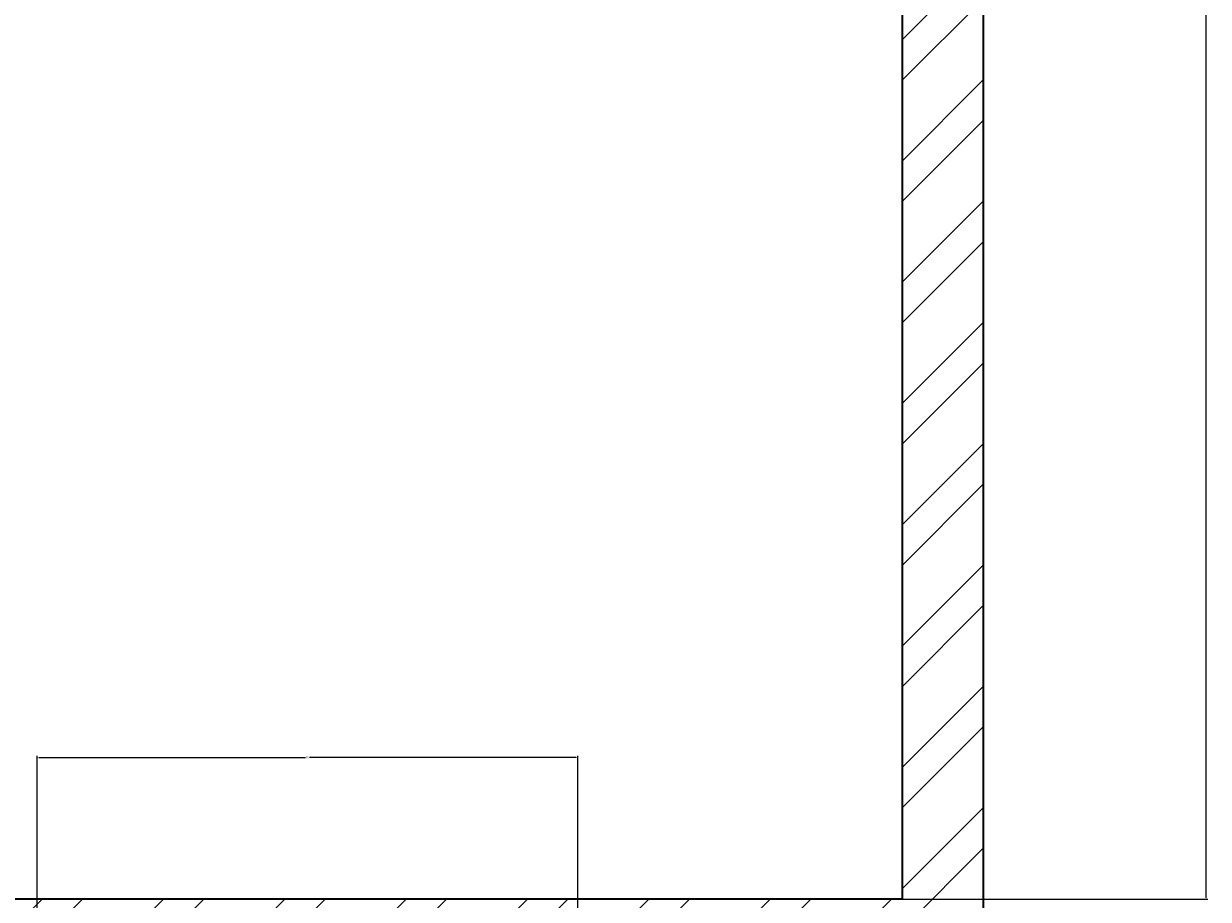
# Model space of a CAD drawing. Units: inches. Extents: x 2166 to 3588, y 1959 to 2628.
# Tile 12 of 13: x 3457 to 3588, y 2112 to 2209. Entities that reach past the tile are written whole.
import ezdxf

# ---------------------------------------------------------------- set-up
doc = ezdxf.new("R2010")
doc.units = ezdxf.units.IN
for name, color, linetype, lineweight in [('A-ANNO-DIMS', 2, 'Continuous', 18), ('A-WALL-PATT', 20, 'Continuous', 13), ('WALL', 40, 'Continuous', 35)]:
    doc.layers.add(name, color=color, linetype=linetype, lineweight=lineweight)
doc.styles.get("Standard").update_dxf_attribs({"font": 'arial.ttf'})
doc.dimstyles.get("Standard").update_dxf_attribs({"dimtxt": 0.18, "dimasz": 0.18, "dimexe": 0.18, "dimexo": 0.0625, "dimgap": 0.09, "dimtad": 0, "dimtih": 1, "dimtoh": 1, "dimdec": 4, "dimzin": 0, "dimdsep": 46, "dimtxsty": 'Standard', "dimcen": 0.09, "dimadec": 0, "dimazin": 0, "dimtfac": 1, "dimtdec": 4, "dimtofl": 0, "dimtmove": 0, "dimatfit": 3, "dimfxl": 1, "dimtolj": 1, "dimtzin": 0, "dimarcsym": 0})

# ---------------------------------------------------------------- blocks, each defined once
blk = doc.blocks.new('*D49')
at = {"layer": 'A-ANNO-DIMS', "color": 0, "lineweight": -2, "transparency": 16777216}
for p, q in [((3554.53, 2420.98), (3588.4, 2420.98)), ((3588.22, 2420.8), (3588.22, 2266.66)), ((3588.22, 2112.16), (3588.22, 2266.3)), ((3554.53, 2111.98), (3588.4, 2111.98))]:
    blk.add_line(p, q, dxfattribs=at)
at = {"layer": 'A-ANNO-DIMS', "color": 0, "transparency": 16777216}
for points in [[(3588.19, 2420.8), (3588.25, 2420.8), (3588.22, 2420.98)], [(3588.19, 2112.16), (3588.25, 2112.16), (3588.22, 2111.98)]]:
    blk.add_solid(points, dxfattribs=at)
at = {"layer": 'Defpoints', "color": 0, "transparency": 16777216}
for p in [(3554.47, 2420.98), (3588.22, 2420.98), (3554.47, 2111.98)]:
    blk.add_point(p, dxfattribs=at)
at = {"layer": 'A-ANNO-DIMS', "color": 0, "transparency": 16777216, "insert": (3588.22, 2266.48), "char_height": 0.18, "attachment_point": 5}
blk.add_mtext('\\A1;309', dxfattribs=at)
blk = doc.blocks.new('*D52')
at = {"layer": 'A-ANNO-DIMS', "color": 0, "lineweight": -2, "transparency": 16777216}
for p, q in [((3458.47, 2103.04), (3458.47, 2127.91)), ((3458.65, 2127.73), (3488.25, 2127.73)), ((3518.29, 2127.73), (3488.69, 2127.73)), ((3518.47, 2103.04), (3518.47, 2127.91))]:
    blk.add_line(p, q, dxfattribs=at)
at = {"layer": 'A-ANNO-DIMS', "color": 0, "transparency": 16777216}
for points in [[(3458.65, 2127.76), (3458.65, 2127.7), (3458.47, 2127.73)], [(3518.29, 2127.76), (3518.29, 2127.7), (3518.47, 2127.73)]]:
    blk.add_solid(points, dxfattribs=at)
at = {"layer": 'Defpoints', "color": 0, "transparency": 16777216}
for p in [(3518.47, 2127.73), (3458.47, 2102.98), (3518.47, 2102.98)]:
    blk.add_point(p, dxfattribs=at)
at = {"layer": 'A-ANNO-DIMS', "color": 0, "transparency": 16777216, "insert": (3488.47, 2127.73), "char_height": 0.18, "attachment_point": 5}
blk.add_mtext('\\A1;60', dxfattribs=at)

msp = doc.modelspace()

# ---------------------------------------------------------------- hatches: boundary and pattern name
at = {"layer": 'A-WALL-PATT'}
h = msp.add_hatch(dxfattribs=at)
h.set_pattern_fill('ANSI32', color=256)
h.paths.add_polyline_path([(3563.471, 2429.979), (3227.471, 2429.979), (3227.471, 2021.979), (3563.471, 2021.979)])
h.paths.add_polyline_path([(3236.471, 2420.979), (3554.471, 2420.979), (3554.471, 2111.979), (3236.471, 2111.979)], flags=16)
h.paths.add_polyline_path([(3236.471, 2102.979), (3554.471, 2102.979), (3554.471, 2030.979), (3236.471, 2030.979)], flags=16)
h.paths.add_polyline_path([(3518.471, 2085.283), (3518.471, 2067.979), (3458.471, 2067.979), (3458.471, 2085.283)], flags=0)
h.paths.add_polyline_path([(3434.656, 2082.283), (3442.194, 2082.283), (3442.194, 2087.514), (3434.656, 2087.514)], flags=8)
h.paths.add_polyline_path([(3522.671, 2094.512), (3521.752, 2052.984), (3545.541, 2052.457), (3546.46, 2093.986)], flags=8)

# ---------------------------------------------------------------- linework, layer by layer
at = {"layer": 'WALL'}
msp.add_line((3554.471, 2111.979), (3236.471, 2111.979), dxfattribs=at)
msp.add_lwpolyline([(3227.471, 2429.979), (3563.471, 2429.979), (3563.471, 2021.979), (3227.471, 2021.979)], close=True, dxfattribs=at)
msp.add_lwpolyline([(3236.471, 2111.979), (3236.471, 2420.979), (3554.471, 2420.979), (3554.471, 2111.979)], dxfattribs=at)

# ---------------------------------------------------------------- dimensions: what is measured, and where the dimension line sits
at = {"layer": 'A-ANNO-DIMS'}
dim = msp.add_linear_dim(base=(3588.221, 2420.979), p1=(3554.471, 2111.979), p2=(3554.471, 2420.979), angle=90, dimstyle='Standard', override={"dimdec": 0, "dimlfac": 1, "dimrnd": 0, "dimzin": 0, "dimdsep": 46, "dimlunit": 2}, dxfattribs=at)
dim.commit()
dim.dimension.update_dxf_attribs({"geometry": '*D49', "text_midpoint": (3588.221, 2266.479)})
dim = msp.add_linear_dim(base=(3518.471, 2127.729), p1=(3458.471, 2102.979), p2=(3518.471, 2102.979), dimstyle='Standard', override={"dimdec": 0, "dimlfac": 1, "dimrnd": 0, "dimzin": 0, "dimdsep": 46, "dimlunit": 2}, dxfattribs=at)
dim.commit()
dim.dimension.update_dxf_attribs({"geometry": '*D52', "text_midpoint": (3488.471, 2127.729)})

doc.saveas('drawing.dxf')
